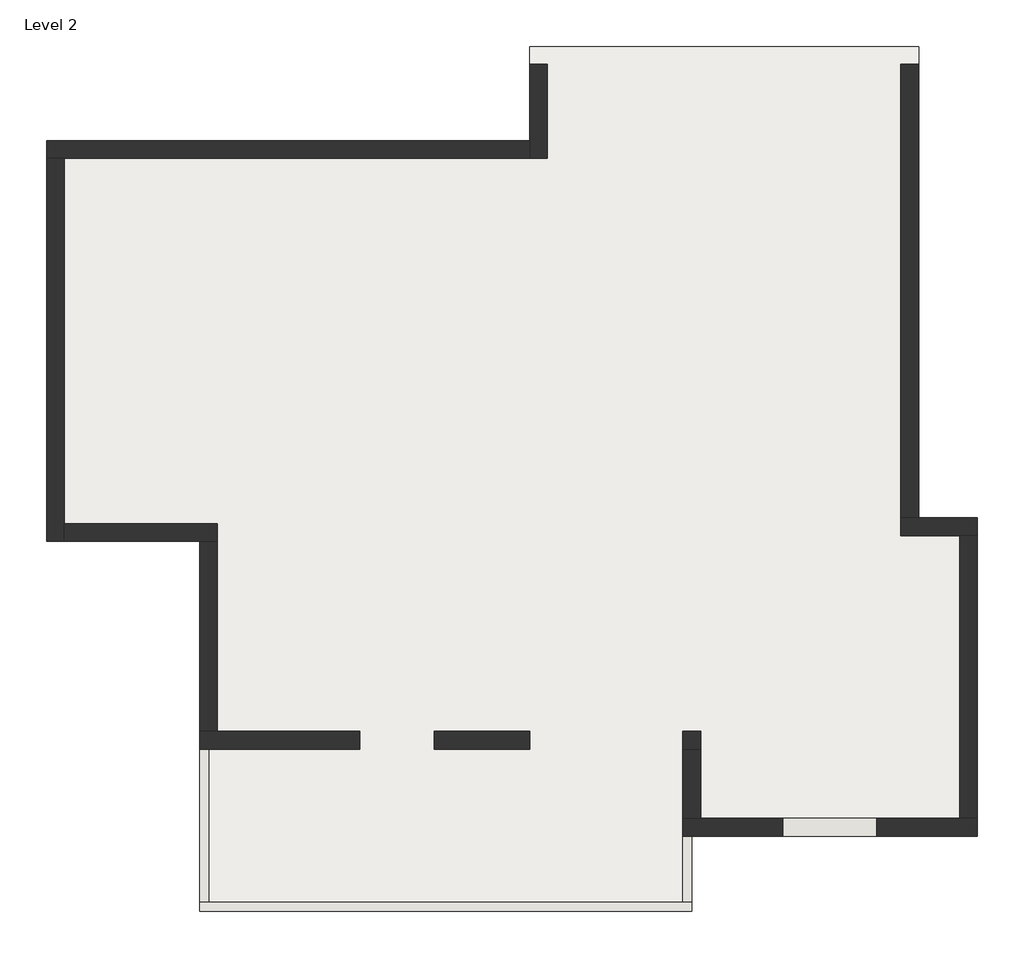
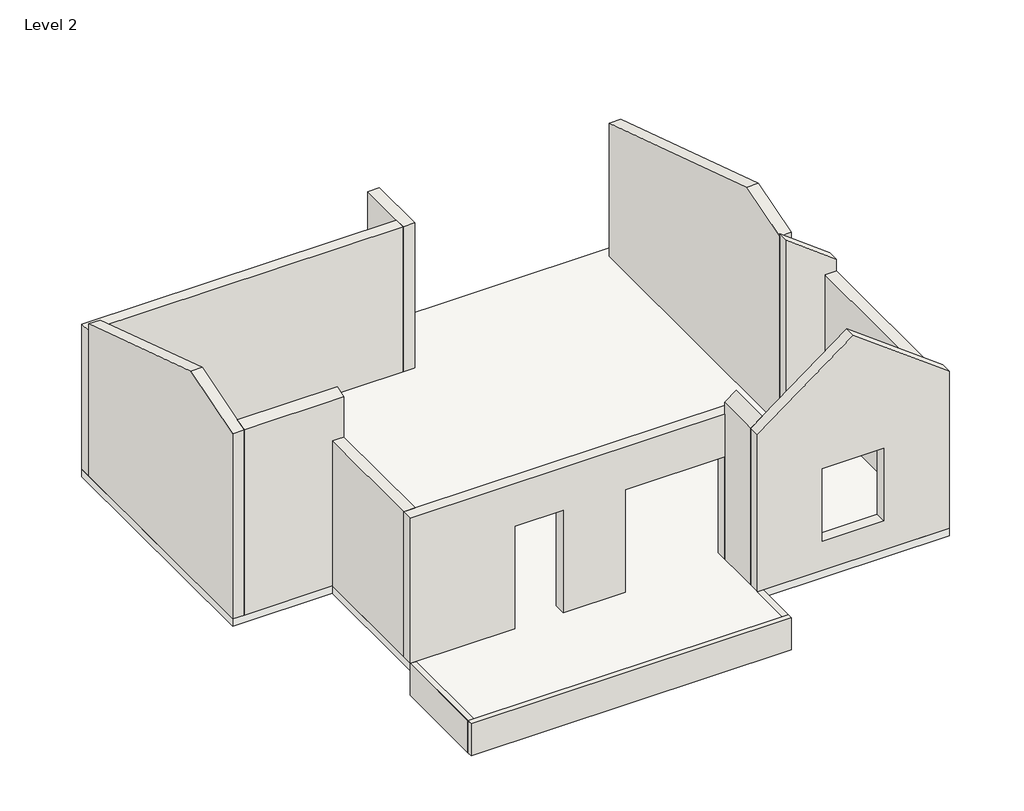
# One storey: 14 walls, 1 roof.
"""IFC4 building model written with IfcOpenShell, lengths in millimetres."""

from ifc_helpers import new_model, si_unit, frame, origin, place, context, project, spatial, polyline, outline, extrude, faceted_brep, element, save

model = new_model("IFC4")

# Units and contexts
model_context = context("Model", 3, world=origin())
ifc_project = project(units=[si_unit("LENGTHUNIT", "METRE", prefix="MILLI")], contexts=[model_context])

# Site, building, storey
site = spatial("IfcSite", under=ifc_project)
building = spatial("IfcBuilding", under=site)
storey = spatial("IfcBuildingStorey", under=building, Name="Level 2", Elevation=3048.0)

# Roof
placement = place(None, origin())
element("IfcRoof", 1, ObjectType="6\" roof", at=placement, inside=storey, context=model_context, shape_type="SweptSolid", body=[
    extrude(outline(polyline([(-7863.8915113, 4174.3099631), (-9845.0915113, 4174.3099631), (-9845.0915113, 9355.9099631), (-3596.6915113, 9355.9099631), (-3596.6915113, 10575.1099631), (1432.5084887, 10575.1099631), (1432.5084887, 4479.1099631), (2194.5084887, 4479.1099631), (2194.5084887, 364.3099631), (-1501.1915113, 364.3099631), (-1501.1915113, -606.4728083), (-7863.8915113, -606.4728083), (-7863.8915113, 4174.3099631)])), frame((0.0, 0.0, 3048.0), z_axis=(0.0, 0.0, 1.0), x_axis=(1.0, 0.0, 0.0)), (0.0, 0.0, 1.0), 152.4),
])

# Walls
element("IfcWall", 2, ObjectType="4.5\" wall", at=placement, inside=storey, context=model_context, shape_type="Brep", body=[
    faceted_brep([(-1501.1915113, -492.1728083, 2530.5713747), (-1615.4915113, -492.1728083, 2530.5713747), (-7749.5915113, -492.1728083, 2530.5713747), (-7863.8915113, -492.1728083, 2530.5713747), (-7863.8915113, -492.1728083, 3200.4), (-7749.5915113, -492.1728083, 3200.4), (-1615.4915113, -492.1728083, 3200.4), (-1501.1915113, -492.1728083, 3200.4), (-1501.1915113, -606.4728083, 2530.5713747), (-1501.1915113, -606.4728083, 3200.4), (-7863.8915113, -606.4728083, 3200.4), (-7863.8915113, -606.4728083, 2530.5713747)], [[[0, 1, 2, 3, 4, 5, 6, 7]], [[8, 9, 10, 11]], [[0, 7, 9, 8]], [[4, 3, 11, 10]], [[3, 2, 1, 0, 8, 11]], [[7, 6, 5, 4, 10, 9]]]),
])
element("IfcWall", 3, ObjectType="4.5\" wall", at=placement, inside=storey, context=model_context, shape_type="Brep", body=[
    faceted_brep([(-7749.5915113, -492.1728083, 2530.5713747), (-7749.5915113, 1488.2599631, 2530.5713747), (-7749.5915113, 1488.2599631, 3200.4), (-7749.5915113, -492.1728083, 3200.4), (-7863.8915113, -492.1728083, 2530.5713747), (-7863.8915113, -492.1728083, 3200.4), (-7863.8915113, 1488.2599631, 3200.4), (-7863.8915113, 1488.2599631, 3048.0), (-7863.8915113, 1488.2599631, 2530.5713747)], [[[0, 1, 2, 3]], [[4, 5, 6, 7, 8]], [[1, 0, 4, 8]], [[3, 2, 6, 5]], [[2, 1, 8, 7, 6]], [[0, 3, 5, 4]]]),
])
element("IfcWall", 4, ObjectType="4.5\" wall", at=placement, inside=storey, context=model_context, shape_type="Brep", body=[
    faceted_brep([(-1501.1915113, -492.1728083, 2530.5713747), (-1501.1915113, 364.3099631, 2530.5713747), (-1501.1915113, 364.3099631, 3200.4), (-1501.1915113, -492.1728083, 3200.4), (-1615.4915113, -492.1728083, 2530.5713747), (-1615.4915113, -492.1728083, 3200.4), (-1615.4915113, 364.3099631, 3200.4), (-1615.4915113, 364.3099631, 3048.0), (-1615.4915113, 364.3099631, 2530.5713747)], [[[0, 1, 2, 3]], [[4, 5, 6, 7, 8]], [[1, 0, 4, 8]], [[3, 2, 6, 5]], [[2, 1, 8, 7, 6]], [[0, 3, 5, 4]]]),
])
element("IfcWall", 5, ObjectType="9\" wall", at=placement, inside=storey, context=model_context, shape_type="Brep", body=[
    faceted_brep([(-7863.8915113, 1716.8599631, 6248.4), (-7635.2915113, 1716.8599631, 6248.4), (-1386.8915113, 1716.8599631, 6248.4), (-1386.8915113, 1716.8599631, 3200.4), (-1615.4915113, 1716.8599631, 3200.4), (-1615.4915113, 1716.8599631, 5359.4), (-3596.6915113, 1716.8599631, 5359.4), (-3596.6915113, 1716.8599631, 3200.4), (-4828.5915113, 1716.8599631, 3200.4), (-4828.5915113, 1716.8599631, 5359.4), (-5793.7915113, 1716.8599631, 5359.4), (-5793.7915113, 1716.8599631, 3200.4), (-7635.2915113, 1716.8599631, 3200.4), (-7863.8915113, 1716.8599631, 3200.4), (-1386.8915113, 1488.2599631, 6248.4), (-7863.8915113, 1488.2599631, 6248.4), (-7863.8915113, 1488.2599631, 3200.4), (-5793.7915113, 1488.2599631, 3200.4), (-5793.7915113, 1488.2599631, 5359.4), (-4828.5915113, 1488.2599631, 5359.4), (-4828.5915113, 1488.2599631, 3200.4), (-3596.6915113, 1488.2599631, 3200.4), (-3596.6915113, 1488.2599631, 5359.4), (-1615.4915113, 1488.2599631, 5359.4), (-1615.4915113, 1488.2599631, 3200.4), (-1386.8915113, 1488.2599631, 3200.4)], [[[0, 1, 2, 3, 4, 5, 6, 7, 8, 9, 10, 11, 12, 13]], [[14, 15, 16, 17, 18, 19, 20, 21, 22, 23, 24, 25]], [[16, 13, 12, 11, 17]], [[3, 25, 24, 4]], [[20, 8, 7, 21]], [[2, 1, 0, 15, 14]], [[0, 13, 16, 15]], [[3, 2, 14, 25]], [[19, 9, 8, 20]], [[9, 19, 18, 10]], [[10, 18, 17, 11]], [[23, 5, 4, 24]], [[5, 23, 22, 6]], [[6, 22, 21, 7]]]),
])
element("IfcWall", 6, ObjectType="9\" wall", at=placement, inside=storey, context=model_context, shape_type="Brep", body=[
    faceted_brep([(2194.5084887, 592.9099631, 3200.4), (1965.9084887, 592.9099631, 3200.4), (-1386.8915113, 592.9099631, 3200.4), (-1615.4915113, 592.9099631, 3200.4), (-1615.4915113, 592.9099631, 6496.05), (-1386.8915113, 592.9099631, 6667.5), (289.5084887, 592.9099631, 7924.8), (2194.5084887, 592.9099631, 6496.05), (2194.5084887, 592.9099631, 6248.4), (892.7584887, 592.9099631, 3810.0), (892.7584887, 592.9099631, 5334.0), (-326.4415113, 592.9099631, 5334.0), (-326.4415113, 592.9099631, 3810.0), (-1615.4915113, 364.3099631, 3200.4), (2194.5084887, 364.3099631, 3200.4), (2194.5084887, 364.3099631, 6496.05), (289.5084887, 364.3099631, 7924.8), (-1615.4915113, 364.3099631, 6496.05), (892.7584887, 364.3099631, 5334.0), (892.7584887, 364.3099631, 3810.0), (-326.4415113, 364.3099631, 3810.0), (-326.4415113, 364.3099631, 5334.0)], [[[0, 1, 2, 3, 4, 5, 6, 7, 8], [9, 10, 11, 12]], [[13, 14, 15, 16, 17], [18, 19, 20, 21]], [[3, 2, 1, 0, 14, 13]], [[4, 3, 13, 17]], [[0, 8, 7, 15, 14]], [[9, 19, 18, 10]], [[10, 18, 21, 11]], [[11, 21, 20, 12]], [[19, 9, 12, 20]], [[15, 7, 6, 16]], [[4, 17, 16, 6, 5]]]),
])
element("IfcWall", 7, ObjectType="9\" wall", at=placement, inside=storey, context=model_context, shape_type="Brep", body=[
    faceted_brep([(-1386.8915113, 592.9099631, 3200.4), (-1386.8915113, 1488.2599631, 3200.4), (-1386.8915113, 1488.2599631, 6248.4), (-1386.8915113, 1488.2599631, 6667.5), (-1386.8915113, 592.9099631, 6667.5), (-1615.4915113, 592.9099631, 3200.4), (-1615.4915113, 592.9099631, 6496.05), (-1615.4915113, 1488.2599631, 6496.05), (-1615.4915113, 1488.2599631, 3200.4)], [[[0, 1, 2, 3, 4]], [[5, 6, 7, 8]], [[1, 0, 5, 8]], [[3, 2, 1, 8, 7]], [[0, 4, 6, 5]], [[4, 3, 7, 6]]]),
])
element("IfcWall", 8, ObjectType="9\" wall", at=placement, inside=storey, context=model_context, shape_type="SweptSolid", body=[
    extrude(outline(polyline([(1965.9084887, 592.9099631), (1965.9084887, 4250.5099631), (2194.5084887, 4250.5099631), (2194.5084887, 592.9099631), (1965.9084887, 592.9099631)])), frame((0.0, 0.0, 3200.4), z_axis=(0.0, 0.0, 1.0), x_axis=(1.0, 0.0, 0.0)), (0.0, 0.0, 1.0), 3048.0),
])
element("IfcWall", 9, ObjectType="9\" wall", at=placement, inside=storey, context=model_context, shape_type="Brep", body=[
    faceted_brep([(1203.9084887, 4250.5099631, 3200.4), (1965.9084887, 4250.5099631, 3200.4), (2194.5084887, 4250.5099631, 3200.4), (2194.5084887, 4250.5099631, 6248.4), (2194.5084887, 4250.5099631, 6496.05), (1203.9084887, 4250.5099631, 7239.0), (1203.9084887, 4479.1099631, 3200.4), (1203.9084887, 4479.1099631, 7187.6937607), (1203.9084887, 4479.1099631, 7239.0), (2194.5084887, 4479.1099631, 6496.05), (2194.5084887, 4479.1099631, 3200.4), (1432.5084887, 4479.1099631, 3200.4)], [[[0, 1, 2, 3, 4, 5]], [[6, 7, 8, 9, 10, 11]], [[2, 1, 0, 6, 11, 10]], [[4, 3, 2, 10, 9]], [[0, 5, 8, 7, 6]], [[5, 4, 9, 8]]]),
])
element("IfcWall", 10, ObjectType="9\" wall", at=placement, inside=storey, context=model_context, shape_type="SweptSolid", body=[
    extrude(outline(polyline([(10346.5099631, 3200.4), (4479.1099631, 3200.4), (4479.1099631, 7187.6937607), (5608.4506361, 7532.9678542), (10346.5099631, 6001.9502231), (10346.5099631, 3200.4)])), frame((1203.9084887, 0.0, 0.0), z_axis=(1.0, 0.0, 0.0), x_axis=(0.0, 1.0, 0.0)), (0.0, 0.0, 1.0), 228.6),
])
element("IfcWall", 11, ObjectType="9\" wall", at=placement, inside=storey, context=model_context, shape_type="Brep", body=[
    faceted_brep([(-3596.6915113, 10346.5099631, 3200.4), (-3596.6915113, 9355.9099631, 3200.4), (-3596.6915113, 9127.3099631, 3200.4), (-3596.6915113, 9127.3099631, 6248.4), (-3596.6915113, 9355.9099631, 6248.4), (-3596.6915113, 10346.5099631, 6248.4), (-3368.0915113, 10346.5099631, 3200.4), (-3368.0915113, 10346.5099631, 6248.4), (-3368.0915113, 9127.3099631, 6248.4), (-3368.0915113, 9127.3099631, 3200.4)], [[[0, 1, 2, 3, 4, 5]], [[6, 7, 8, 9]], [[2, 1, 0, 6, 9]], [[5, 4, 3, 8, 7]], [[3, 2, 9, 8]], [[0, 5, 7, 6]]]),
])
element("IfcWall", 12, ObjectType="9\" wall", at=placement, inside=storey, context=model_context, shape_type="Brep", body=[
    faceted_brep([(-3596.6915113, 9355.9099631, 3200.4), (-9845.0915113, 9355.9099631, 3200.4), (-9845.0915113, 9355.9099631, 6248.4), (-3596.6915113, 9355.9099631, 6248.4), (-3596.6915113, 9127.3099631, 3200.4), (-3596.6915113, 9127.3099631, 6248.4), (-9845.0915113, 9127.3099631, 6248.4), (-9845.0915113, 9127.3099631, 3200.4), (-9616.4915113, 9127.3099631, 3200.4)], [[[0, 1, 2, 3]], [[4, 5, 6, 7, 8]], [[1, 0, 4, 8, 7]], [[3, 2, 6, 5]], [[0, 3, 5, 4]], [[2, 1, 7, 6]]]),
])
element("IfcWall", 13, ObjectType="9\" wall", at=placement, inside=storey, context=model_context, shape_type="Brep", body=[
    faceted_brep([(-9845.0915113, 9127.3099631, 3200.4), (-9845.0915113, 4174.3099631, 3200.4), (-9845.0915113, 4174.3099631, 7094.507049), (-9845.0915113, 5608.4506361, 7532.9678542), (-9845.0915113, 9127.3099631, 6395.9125117), (-9845.0915113, 9127.3099631, 6248.4), (-9616.4915113, 9127.3099631, 3200.4), (-9616.4915113, 9127.3099631, 6395.9125117), (-9616.4915113, 5608.4506361, 7532.9678542), (-9616.4915113, 4402.9099631, 7164.3970828), (-9616.4915113, 4174.3099631, 7094.507049), (-9616.4915113, 4174.3099631, 3200.4), (-9616.4915113, 4402.9099631, 3200.4)], [[[0, 1, 2, 3, 4, 5]], [[6, 7, 8, 9, 10, 11, 12]], [[1, 0, 6, 12, 11]], [[0, 5, 4, 7, 6]], [[2, 1, 11, 10]], [[4, 3, 8, 7]], [[3, 2, 10, 9, 8]]]),
])
element("IfcWall", 14, ObjectType="9\" wall", at=placement, inside=storey, context=model_context, shape_type="Brep", body=[
    faceted_brep([(-9616.4915113, 4174.3099631, 3200.4), (-7863.8915113, 4174.3099631, 3200.4), (-7635.2915113, 4174.3099631, 3200.4), (-7635.2915113, 4174.3099631, 6248.4), (-7635.2915113, 4174.3099631, 7094.507049), (-9616.4915113, 4174.3099631, 7094.507049), (-9616.4915113, 4402.9099631, 3200.4), (-9616.4915113, 4402.9099631, 7164.3970828), (-7635.2915113, 4402.9099631, 7164.3970828), (-7635.2915113, 4402.9099631, 3200.4)], [[[0, 1, 2, 3, 4, 5]], [[6, 7, 8, 9]], [[2, 1, 0, 6, 9]], [[0, 5, 7, 6]], [[4, 3, 2, 9, 8]], [[5, 4, 8, 7]]]),
])
element("IfcWall", 15, ObjectType="9\" wall", at=placement, inside=storey, context=model_context, shape_type="SweptSolid", body=[
    extrude(outline(polyline([(-7863.8915113, 1716.8599631), (-7863.8915113, 4174.3099631), (-7635.2915113, 4174.3099631), (-7635.2915113, 1716.8599631), (-7863.8915113, 1716.8599631)])), frame((0.0, 0.0, 3200.4), z_axis=(0.0, 0.0, 1.0), x_axis=(1.0, 0.0, 0.0)), (0.0, 0.0, 1.0), 3048.0),
])

save(model, "model.ifc")

# Revit data of these elements
# Type "6\" roof"
#   Assembly Code = "B1020"
#   Layers, outside or top first: 0' - 6" "Laminate, Ivory, Matte" (function 1)
# Type "4.5\" wall"
#   Assembly Code = "B2010"
#   Layers, outside or top first: 0' - 4 1/2" "Laminate, Ivory, Matte" (function 1)
# Type "9\" wall"
#   Assembly Code = "B2010"
#   Layers, outside or top first: 0' - 9" "Laminate, Ivory, Matte" (function 1)
# Element 1 (IfcRoof, "6\" roof")
#   built-in parameter 1001705 = 10.5 (stored number, unit not read)
#   built-in parameter 1001710 = 33615
#   Phase Created = New Construction
#   Materials on its faces: "Laminate, Ivory, Matte"
# Elements 2, 3, 4 (IfcWall, "4.5\" wall")
#   built-in parameter 1001111 = -1' - 8.37121"
#   Top Offset = 0' - 0"
#   Base Offset = -1' - 8.37121"
#   wall height = 2' - 2.37121"
#   Phase Created = New Construction
#   Base Constraint = Level 2
#   Top Constraint = Level 3
#   Materials on its faces: "Laminate, Ivory, Matte"
# Elements 5, 6, 7, 8, 9, 10, 11, 12, 13, 14, 15 (IfcWall, "9\" wall")
#   built-in parameter 1001111 = 0' - 6"
#   Top Offset = 10' - 0"
#   Base Offset = 0' - 6"
#   wall height = 10' - 0"
#   Phase Created = New Construction
#   Base Constraint = Level 2
#   Top Constraint = Level 3
#   Materials on its faces: "Laminate, Ivory, Matte"
# Materials
#   "Laminate, Ivory, Matte": class "Plastic", colour RGB 247 247 239, transparency 0, Description = "Plastic Laminate - Ivory, Matte", Cost = 0
